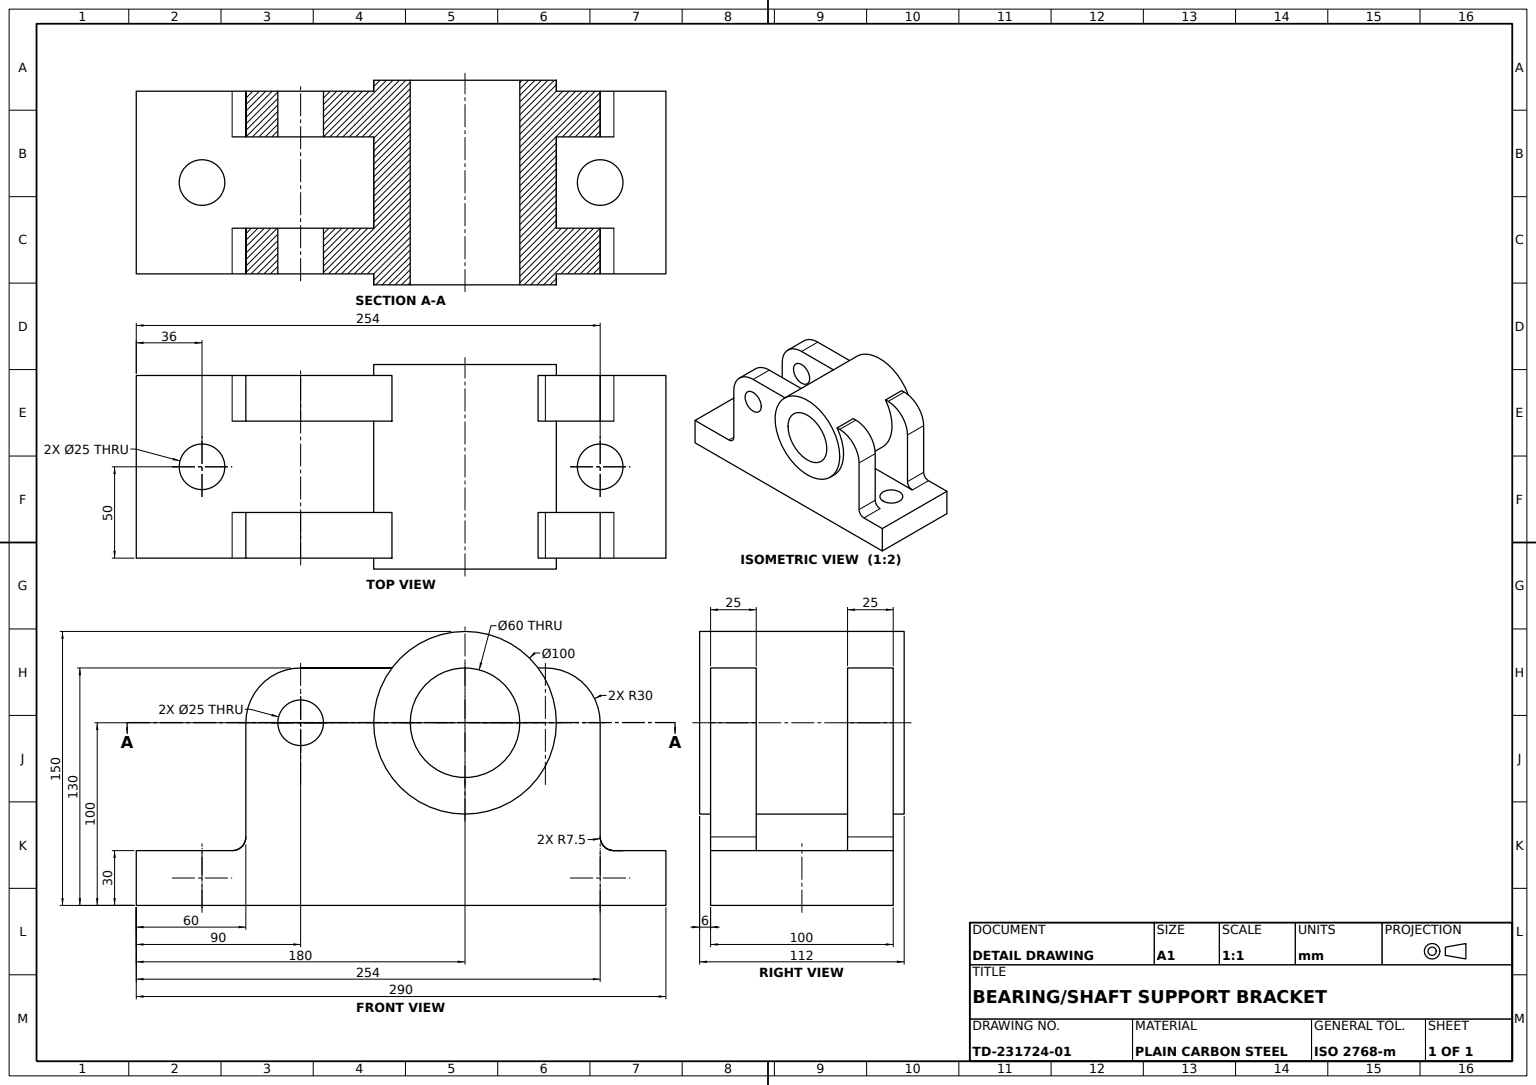
SolidWorks part; units mm, degrees
material "Plain Carbon Steel"
ref_plane "Front Plane" through (0, 0, 0) normal (0, 0, 1) x (1, 0, 0)
ref_plane "Top Plane" through (0, 0, 0) normal (0, 1, 0) x (1, 0, 0)
ref_plane "Right Plane" through (0, 0, 0) normal (1, 0, 0) x (0, 0, -1)
sketch "Base Plate Sketch" plane through (0, 0, 0) normal (0, 0, 1) x (1, 0, 0)
  line L0 (210.6769, 0) -> (-274.4533, 0) construction
  line L1 (0, -212.1101) -> (0, 240.0571) construction
  line L2 (-180, 0) -> (-180, 30)
  line L3 (-180, 0) -> (110, 0)
  line L4 (110, 0) -> (110, 30)
  line L5 (110, 30) -> (-180, 30)
  dimension "D1" = 290
  dimension "D2" = 30
  dimension "D3" = 180
extrude "Base Plate" add sketch "Base Plate Sketch" along normal mid plane 100
sketch "Bearing Boss Sketch" plane through (0, 0, 0) normal (0, 0, 1) x (1, 0, 0)
  line L0 (0, -57.8057) -> (0, 129.734) construction
  line L1 (110, 30) -> (-180, 30) construction
  circle A0 centre (0, 100) radius 50
  circle A1 centre (0, 100) radius 30
  dimension "D1" = 100
  dimension "D3" = 60
  dimension "D2" = 70
extrude "Bearing Boss" add sketch "Bearing Boss Sketch" along normal mid plane 112 separate body
sketch "Base Mounting Cut Sketch" plane through (0, 0, 0) normal (0, 1, 0) x (1, 0, 0)
  line L1 (145.5693, 0) -> (-219.701, 0) construction
  line L2 (-180, -50) -> (-180, 50) construction
  line L3 (110, -50) -> (110, 50) construction
  circle A1 centre (-144, 0) radius 12.5
  circle A2 centre (74, 0) radius 12.5
  dimension "D1" = 25
  dimension "D3" = 25
  dimension "D2" = 36
  dimension "D4" = 36
extrude "Base Mounting Cut" cut sketch "Base Mounting Cut Sketch" against normal mid plane 112
sketch "Support Lug Sketch" plane through (0, 0, 0) normal (0, 1, 0) x (1, 0, 0)
  line L0 (-120, -50) -> (-120, -25)
  line L1 (110, -50) -> (-180, -50) construction
  line L2 (-180, -50) -> (-180, 50) construction
  line L3 (-120, -25) -> (74, -25)
  line L4 (74, -25) -> (74, -50)
  line L5 (74, -50) -> (-120, -50)
  dimension "D1" = 25
  dimension "D2" = 60
  dimension "D3" = 194
extrude "Support Lug" add sketch "Support Lug Sketch" along normal blind 130
mirror "Support Lug Mirror" about plane through (0, 0, 0) normal (0, 0, 1) of "Support Lug"
sketch "Lug Pin Hole Sketch" plane through (0, 0, 0) normal (0, 0, 1) x (1, 0, 0)
  line L0 (-180, 0) -> (110, 0) construction
  line L1 (-120, 130) -> (-120, 30) construction
  circle A0 centre (-90, 100) radius 12.5
  dimension "D1" = 25
  dimension "D2" = 100
  dimension "D3" = 30
extrude "Lug Pin Hole Ø25" cut sketch "Lug Pin Hole Sketch" against normal mid plane 130
sketch "Lug Profile Cut Sketch" plane through (0, 0, 50) normal (0, 0, 1) x (1, 0, 0)
  line L0 (-120, 100) -> (-120, 130)
  line L1 (-120, 130) -> (-90, 130)
  arc A0 (-90, 130) -> (-120, 100) centre (-90, 100) ccw
  dimension "D1" = 60
extrude "Lug Profile Cut" cut sketch "Lug Profile Cut Sketch" against normal blind 130
sketch "Housing Clearance Reference Sketch" plane through (0, 0, 0) normal (0, 0, 1) x (1, 0, 0)
  line L1 (74, 130) -> (74, 30) construction
  line L2 (40, 130) -> (74, 130) construction
  circle A2 centre (44, 100) radius 30
  dimension "D1" = 60
sketch "Housing Clearance Sketch" plane through (0, 0, 50) normal (0, 0, 1) x (1, 0, 0)
  line L0 (44, 130) -> (74, 130)
  line L9 (-40, 130) -> (-90, 130)
  line L10 (-120, 100) -> (-120, 30)
  line L11 (-120, 30) -> (-180, 30)
  line L12 (-180, 30) -> (-180, 0)
  line L13 (-180, 0) -> (110, 0)
  line L14 (110, 0) -> (110, 30)
  line L15 (110, 30) -> (74, 30)
  line L16 (74, 30) -> (74, 130)
  line L17 (74, 130) -> (40, 130)
  line L18 (-40, 130) -> (-90, 130)
  line L19 (-120, 100) -> (-120, 30)
  line L20 (-120, 30) -> (-180, 30)
  line L21 (-180, 30) -> (-180, 0)
  line L22 (-180, 0) -> (110, 0)
  line L23 (110, 0) -> (110, 30)
  line L24 (110, 30) -> (74, 30)
  line L25 (74, 30) -> (74, 130)
  line L26 (74, 130) -> (44, 130)
  circle A0 centre (44, 100) radius 30 construction
  arc A1 (74, 100) -> (44, 130) centre (44, 100) ccw
  arc A2 (-90, 130) -> (-120, 100) centre (-90, 100) ccw
  arc A3 (-40, 130) -> (40, 130) centre (0, 100) ccw
  arc A4 (-90, 130) -> (-120, 100) centre (-90, 100) ccw
  arc A5 (-40, 130) -> (40, 130) centre (0, 100) ccw
  dimension "D1" = 0
extrude "Housing Clearance Cut" cut sketch "Housing Clearance Sketch" against normal blind 110 contours A1 L25 A0
sketch "Bearing Bore Sketch" plane through (0, 0, 56) normal (0, 0, 1) x (1, 0, 0)
  circle A0 centre (0, 100) radius 30
  dimension "D1" = 60
extrude "Bearing Bore Ø60" cut sketch "Bearing Bore Sketch" against normal blind 120
sketch "Rib 1 Sketch" plane through (0, 0, 50) normal (0, 0, 1) x (1, 0, 0)
  line L0 (-120, 30) -> (-180, 30) construction
  line L1 (-120, 100) -> (-120, 30) construction
  line L2 (-127.5, 25.7628) -> (-127.5, 37.5) construction
  line L3 (-127.5, 37.5) -> (-115.5885, 37.5) construction
  line L4 (-127.5, 30) -> (-120, 30)
  line L5 (-120, 30) -> (-120, 37.5)
  arc A0 (-127.5, 30) -> (-120, 37.5) centre (-127.5, 37.5) ccw
  dimension "D1" = 15
extrude "Rib 1" add sketch "Rib 1 Sketch" against normal blind 25
sketch "Rib 2 Sketch" plane through (0, 0, -25) normal (0, 0, 1) x (1, 0, 0)
  line L0 (-127.5, 30) -> (-120, 30)
  line L5 (74, 30) -> (74, 100)
  line L6 (44, 130) -> (40, 130)
  line L7 (-40, 130) -> (-90, 130)
  line L8 (-120, 100) -> (-120, 30)
  line L9 (-120, 30) -> (74, 30)
  line L10 (74, 30) -> (74, 100)
  line L11 (44, 130) -> (40, 130)
  line L12 (-40, 130) -> (-90, 130)
  line L13 (-120, 37.5) -> (-120, 30)
  line L14 (-120, 30) -> (74, 30)
  arc A0 (-127.5, 30) -> (-120, 37.5) centre (-127.5, 37.5) ccw construction
  arc A1 (-127.5, 30) -> (-120, 37.5) centre (-127.5, 37.5) ccw
  arc A3 (74, 100) -> (44, 130) centre (44, 100) ccw
  arc A4 (-40, 130) -> (40, 130) centre (0, 100) ccw
  arc A5 (-90, 130) -> (-120, 100) centre (-90, 100) ccw
  arc A6 (74, 100) -> (44, 130) centre (44, 100) ccw
  arc A7 (-40, 130) -> (40, 130) centre (0, 100) ccw
  arc A8 (-90, 130) -> (-120, 100) centre (-90, 100) ccw
  dimension "D1" = 0
extrude "Rib 2" add sketch "Rib 2 Sketch" against normal blind 25 contours L0 A1 L13
sketch "Rib 3 Sketch" plane through (0, 0, 50) normal (0, 0, 1) x (1, 0, 0)
  line L1 (110, 30) -> (74, 30) construction
  line L2 (74, 100) -> (74, 30) construction
  line L3 (81.5, 37.5) -> (81.5, 21.8997) construction
  line L4 (81.5, 37.5) -> (67.5161, 37.5) construction
  line L5 (74, 37.5) -> (74, 30)
  line L6 (74, 30) -> (81.5, 30)
  arc A0 (74, 37.5) -> (81.5, 30) centre (81.5, 37.5) ccw
  dimension "D1" = 15
extrude "Rib 3" add sketch "Rib 3 Sketch" against normal blind 25
sketch "Rib 4 Sketch" plane through (0, 0, -25) normal (0, 0, 1) x (1, 0, 0)
  line L0 (81.5, 30) -> (74, 30)
  line L5 (74, 30) -> (74, 100)
  line L6 (44, 130) -> (40, 130)
  line L7 (-40, 130) -> (-90, 130)
  line L8 (-120, 100) -> (-120, 37.5)
  line L9 (-127.5, 30) -> (74, 30)
  line L10 (74, 30) -> (74, 100)
  line L11 (44, 130) -> (40, 130)
  line L12 (-40, 130) -> (-90, 130)
  line L13 (-120, 100) -> (-120, 37.5)
  line L14 (-127.5, 30) -> (74, 30)
  arc A0 (74, 37.5) -> (81.5, 30) centre (81.5, 37.5) ccw construction
  arc A1 (74, 37.5) -> (81.5, 30) centre (81.5, 37.5) ccw
  arc A4 (74, 100) -> (44, 130) centre (44, 100) ccw
  arc A5 (-40, 130) -> (40, 130) centre (0, 100) ccw
  arc A6 (-90, 130) -> (-120, 100) centre (-90, 100) ccw
  arc A7 (-127.5, 30) -> (-120, 37.5) centre (-127.5, 37.5) ccw
  arc A8 (74, 100) -> (44, 130) centre (44, 100) ccw
  arc A9 (-40, 130) -> (40, 130) centre (0, 100) ccw
  arc A10 (-90, 130) -> (-120, 100) centre (-90, 100) ccw
  arc A11 (-127.5, 30) -> (-120, 37.5) centre (-127.5, 37.5) ccw
  line M11 (74, 30) -> (74, 100)
  dimension "D1" = 0
extrude "Rib 4" add sketch "Rib 4 Sketch" against normal blind 25 contours A1 L0 M11
